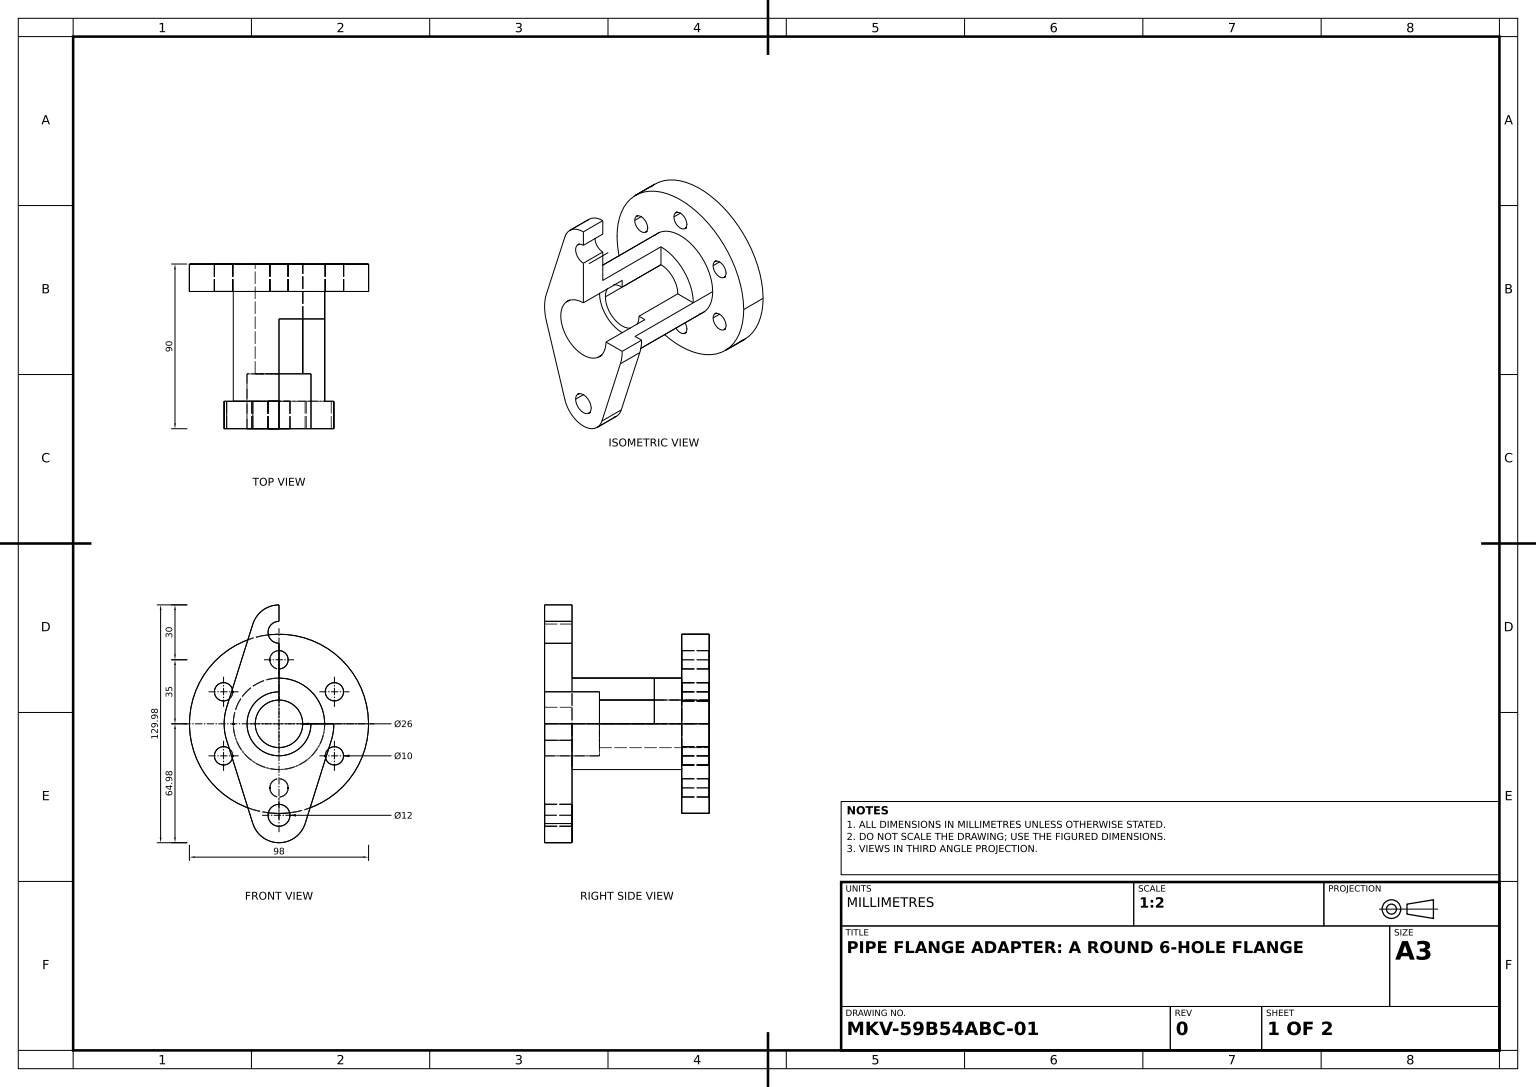
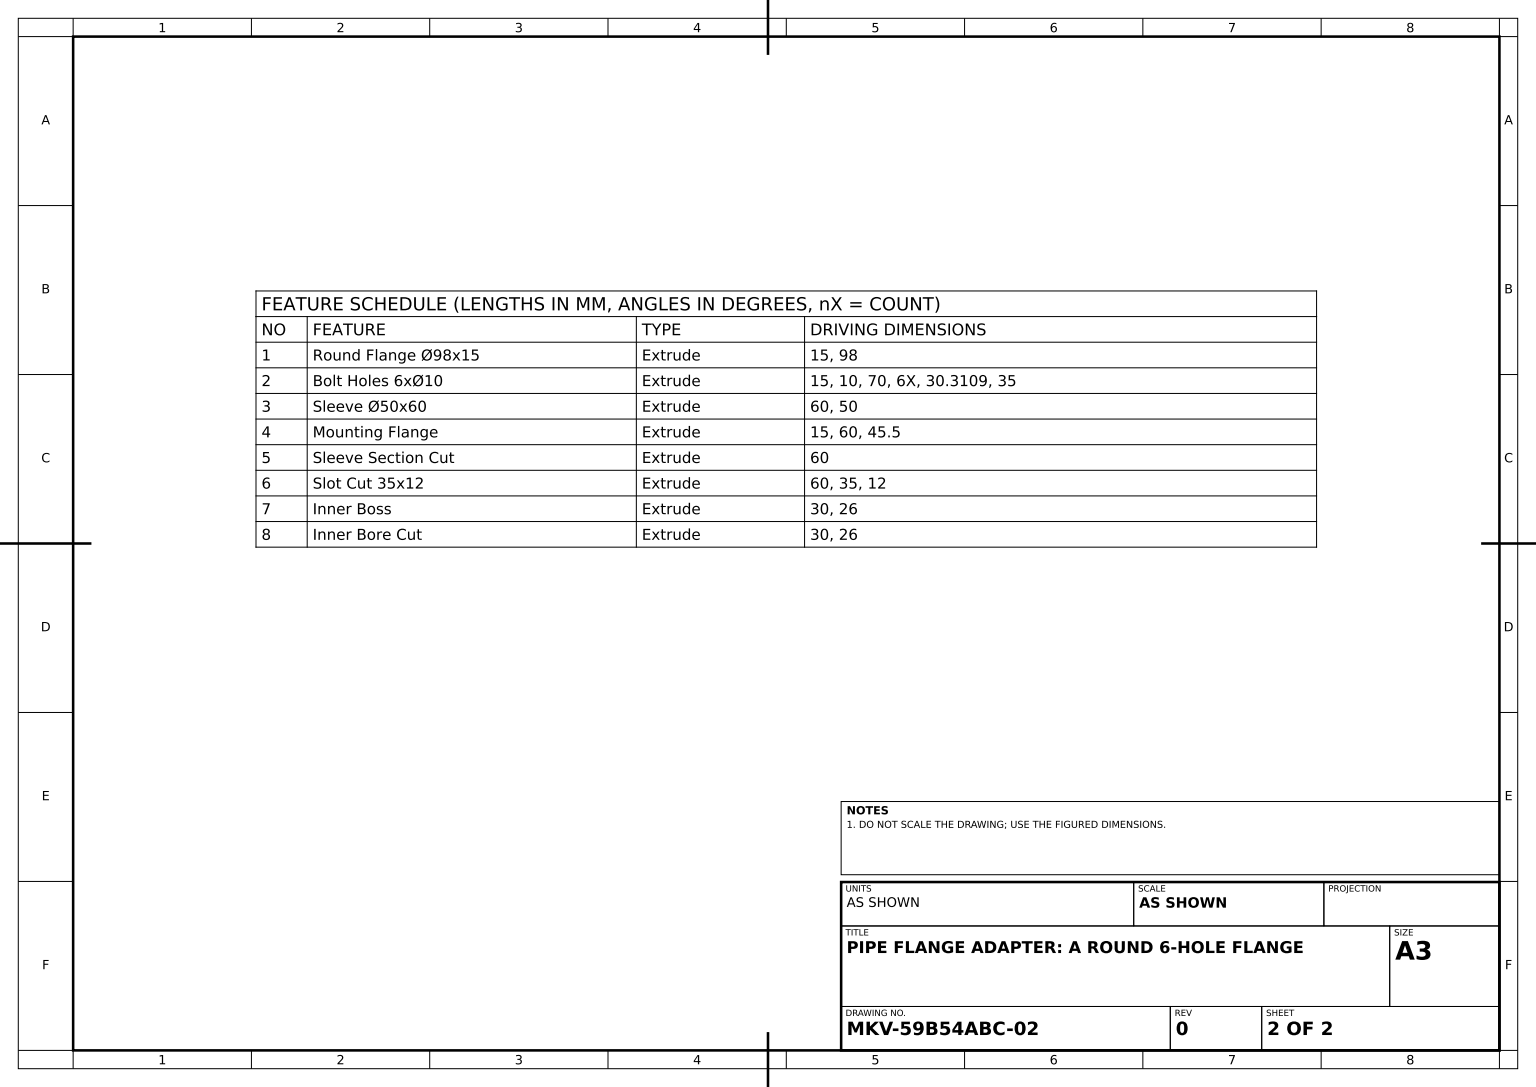
from build123d import *

# Parameters (mm, degrees)
ROUND_FLANGE_SKETCH_98_R        = 49
ROUND_FLANGE_98X15_DEPTH        = 15
BOLT_HOLES_SKETCH_6X_10_PCD70_R = 5
BOLT_HOLES_6X_10_DEPTH          = 15
SLEEVE_SKETCH_50_R              = 25
SLEEVE_50X60_DEPTH              = 60
MOUNTING_FLANGE_DEPTH           = 15
SLEEVE_START                    = -60
SLEEVE_SECTION_CUT_DEPTH        = 60
SLOT_SKETCH_35X12_R             = 17.5
SLOT_SKETCH_35X12_R_2           = 6
SLOT_CUT_35X12_DEPTH            = 60
INNER_START                     = 30
INNER_BOSS_DEPTH                = 30
INNER_BORE_SKETCH_R             = 13
INNER_BORE_CUT_DEPTH            = 30


with BuildPart() as part:
    # Round Flange Sketch Ø98 → Round Flange Ø98x15 (new body)
    with BuildSketch(Plane.XY):
        Circle(ROUND_FLANGE_SKETCH_98_R)
    extrude(amount=-ROUND_FLANGE_98X15_DEPTH)

    # Bolt Holes Sketch 6xØ10 PCD70 → Bolt Holes 6xØ10 (cut)
    with BuildSketch(Plane.XY):
        with Locations((0, 35)):
            Circle(BOLT_HOLES_SKETCH_6X_10_PCD70_R)
        with Locations((30.310889132, 17.5)):
            Circle(BOLT_HOLES_SKETCH_6X_10_PCD70_R)
        with Locations((30.310889132, -17.5)):
            Circle(BOLT_HOLES_SKETCH_6X_10_PCD70_R)
        with Locations((0, -35)):
            Circle(BOLT_HOLES_SKETCH_6X_10_PCD70_R)
        with Locations((-30.310889132, -17.5)):
            Circle(BOLT_HOLES_SKETCH_6X_10_PCD70_R)
        with Locations((-30.310889132, 17.5)):
            Circle(BOLT_HOLES_SKETCH_6X_10_PCD70_R)
    extrude(amount=-BOLT_HOLES_6X_10_DEPTH, mode=Mode.SUBTRACT)

    # Sleeve Sketch Ø50 → Sleeve Ø50x60 (add)
    with BuildSketch(Plane.XY):
        Circle(SLEEVE_SKETCH_50_R)
    extrude(amount=SLEEVE_50X60_DEPTH)

    # Mounting Flange Sketch → Mounting Flange (add)
    with BuildSketch(Plane.XY.offset(60)):
        with BuildLine():
            Line((-28.618176043, -9), (-14.309088021, -54.5))
            ThreePointArc((-14.309088021, -54.5), (0, -65), (14.309088021, -54.5))
            Line((14.309088021, -54.5), (28.618176043, -9))
            ThreePointArc((28.618176043, -9), (30, 0), (28.618176043, 9))
            Line((28.618176043, 9), (14.309088021, 54.5))
            ThreePointArc((14.309088021, 54.5), (0, 65), (-14.309088021, 54.5))
            Line((-14.309088021, 54.5), (-28.618176043, 9))
            ThreePointArc((-28.618176043, 9), (-30, 0), (-28.618176043, -9))
        make_face()
    extrude(amount=MOUNTING_FLANGE_DEPTH)

    # Sleeve Section Cut Sketch → Sleeve Section Cut (cut)
    with BuildSketch(Plane.XY.offset(75).offset(SLEEVE_START)):
        with BuildLine():
            Line((0, 65), (0, 0))
            Line((0, 0), (30, 0))
            ThreePointArc((30, 0), (29.652531774, 4.552730978), (28.618176043, 9))
            Line((28.618176043, 9), (14.309088021, 54.5))
            ThreePointArc((14.309088021, 54.5), (8.874119675, 62.093386622), (0, 65))
        make_face()
    extrude(amount=SLEEVE_SECTION_CUT_DEPTH, mode=Mode.SUBTRACT)

    # Slot Sketch 35x12 → Slot Cut 35x12 (cut)
    with BuildSketch(Plane.XY.offset(75)):
        Circle(SLOT_SKETCH_35X12_R)
        with Locations((0, 50)):
            Circle(SLOT_SKETCH_35X12_R_2)
        with Locations((0, -50)):
            Circle(SLOT_SKETCH_35X12_R_2)
    extrude(amount=-SLOT_CUT_35X12_DEPTH, mode=Mode.SUBTRACT)

    # Inner Boss Sketch → Inner Boss (add)
    with BuildSketch(Plane.XY.offset(15).offset(INNER_START)):
        with BuildLine():
            Line((0, 13), (0, 17.5))
            ThreePointArc((0, 17.5), (-12.374368671, -12.374368671), (17.5, 0))
            Line((17.5, 0), (13, 0))
            ThreePointArc((13, 0), (-9.192388155, -9.192388155), (0, 13))
        make_face()
    extrude(amount=-INNER_BOSS_DEPTH)

    # Inner Bore Sketch → Inner Bore Cut (cut)
    with BuildSketch(Plane.XY.offset(15)):
        Circle(INNER_BORE_SKETCH_R)
    extrude(amount=-INNER_BORE_CUT_DEPTH, mode=Mode.SUBTRACT)


solid = part.part
